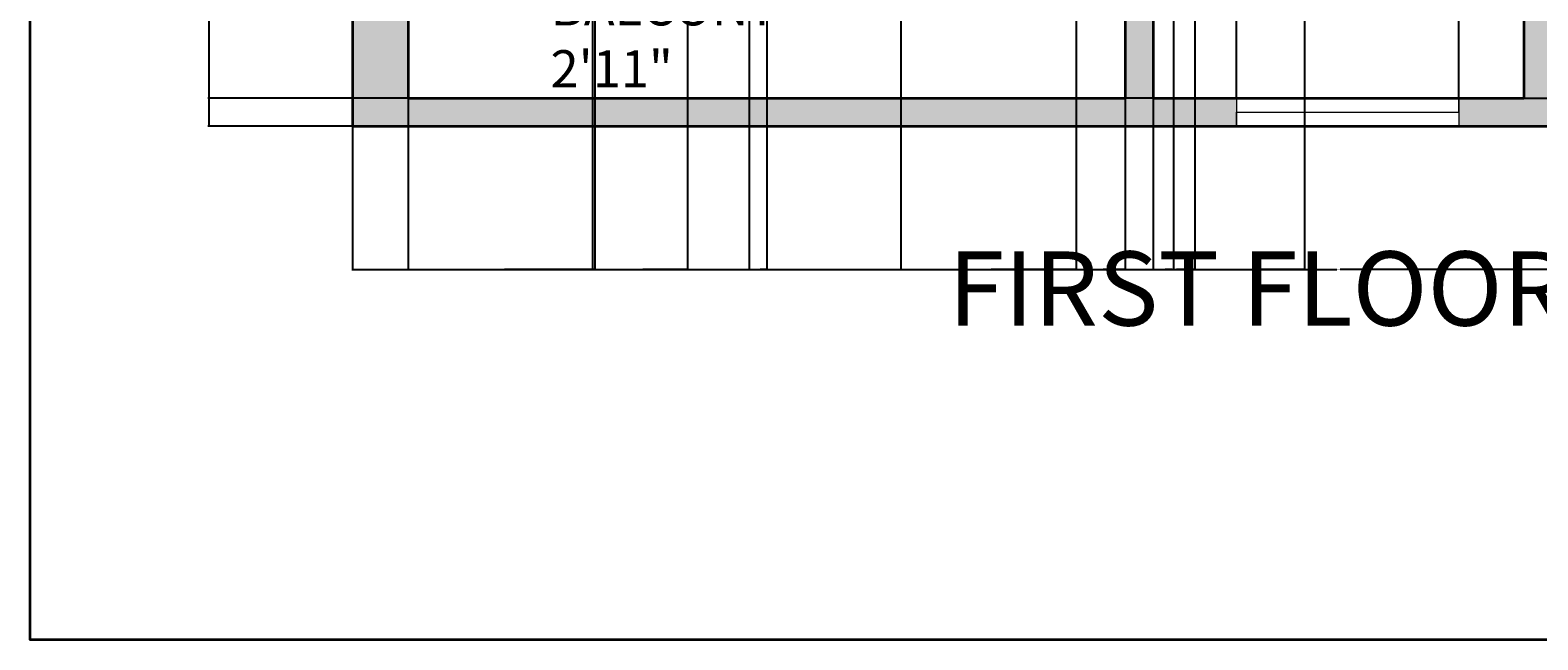
# Model space of a CAD drawing. Units: inches. Extents: x 2606 to 3027, y 1906 to 2463.
# Tile 1 of 10: x 2606 to 2850, y 1906 to 2004. Entities that reach past the tile are written whole.
import ezdxf

# ---------------------------------------------------------------- set-up
doc = ezdxf.new("R2010")
doc.units = ezdxf.units.IN
for name, color, linetype, lineweight in [('A-ANNO-DIMS', 2, 'Continuous', 18), ('A-ANNO-TEXT', 7, 'Continuous', 25), ('A-ANNO-TTLB', 7, 'Continuous', 35), ('A-AREA-IDEN', 7, 'Continuous', 18), ('A-GLAZ', 4, 'Continuous', 18), ('A-WALL', 7, 'Continuous', 35)]:
    doc.layers.add(name, color=color, linetype=linetype, lineweight=lineweight)
doc.layers.add('A-WALL-PATT', color=251, linetype='Continuous', lineweight=13, true_color=0x636466)
doc.styles.get("Standard").update_dxf_attribs({"font": 'arial.ttf'})
doc.dimstyles.get("Standard").update_dxf_attribs({"dimtxt": 0.18, "dimasz": 0.18, "dimexe": 0.18, "dimexo": 0.0625, "dimgap": 0.09, "dimtad": 0, "dimtih": 1, "dimtoh": 1, "dimdec": 4, "dimzin": 0, "dimdsep": 46, "dimtxsty": 'Standard', "dimcen": 0.09, "dimadec": 0, "dimazin": 0, "dimtfac": 1, "dimtdec": 4, "dimtofl": 0, "dimtmove": 0, "dimatfit": 3, "dimfxl": 1, "dimtolj": 1, "dimtzin": 0, "dimarcsym": 0})

# ---------------------------------------------------------------- blocks, each defined once
blk = doc.blocks.new('*D25')
at = {"layer": 'A-ANNO-DIMS', "color": 0, "lineweight": -2, "transparency": 16777216}
for p, q in [((2658.06, 1988.55), (2658.06, 1965.23)), ((2977.06, 1988.55), (2977.06, 1965.23)), ((2658.24, 1965.41), (2817.27, 1965.41)), ((2976.88, 1965.41), (2817.85, 1965.41))]:
    blk.add_line(p, q, dxfattribs=at)
at = {"layer": 'A-ANNO-DIMS', "color": 0, "transparency": 16777216}
for points in [[(2658.24, 1965.44), (2658.24, 1965.38), (2658.06, 1965.41)], [(2976.88, 1965.44), (2976.88, 1965.38), (2977.06, 1965.41)]]:
    blk.add_solid(points, dxfattribs=at)
at = {"layer": 'Defpoints', "color": 0, "transparency": 16777216}
for p in [(2658.06, 1988.61), (2977.06, 1988.61), (2977.06, 1965.41)]:
    blk.add_point(p, dxfattribs=at)
at = {"layer": 'A-ANNO-DIMS', "color": 0, "transparency": 16777216, "insert": (2817.56, 1965.41), "char_height": 0.18, "attachment_point": 5}
blk.add_mtext('\\A1;319', dxfattribs=at)
blk = doc.blocks.new('*D35')
at = {"layer": 'A-ANNO-DIMS', "color": 0, "lineweight": -2, "transparency": 16777216}
for p, q in [((2801.04, 1993.17), (2801.04, 2433.99)), ((2801.22, 2433.81), (2818.82, 2433.81)), ((2836.86, 2433.81), (2819.26, 2433.81)), ((2837.04, 1993.17), (2837.04, 2433.99))]:
    blk.add_line(p, q, dxfattribs=at)
at = {"layer": 'A-ANNO-DIMS', "color": 0, "transparency": 16777216}
for points in [[(2801.22, 2433.84), (2801.22, 2433.78), (2801.04, 2433.81)], [(2836.86, 2433.84), (2836.86, 2433.78), (2837.04, 2433.81)]]:
    blk.add_solid(points, dxfattribs=at)
at = {"layer": 'Defpoints', "color": 0, "transparency": 16777216}
for p in [(2837.04, 2433.81), (2801.04, 1993.11), (2837.04, 1993.11)]:
    blk.add_point(p, dxfattribs=at)
at = {"layer": 'A-ANNO-DIMS', "color": 0, "transparency": 16777216, "insert": (2819.04, 2433.81), "char_height": 0.18, "attachment_point": 5}
blk.add_mtext('\\A1;36', dxfattribs=at)
blk = doc.blocks.new('*D36')
at = {"layer": 'A-ANNO-DIMS', "color": 0, "lineweight": -2, "transparency": 16777216}
for p, q in [((2787.56, 1993.17), (2787.56, 2433.99)), ((2787.74, 2433.81), (2793.85, 2433.81)), ((2800.86, 2433.81), (2794.76, 2433.81)), ((2801.04, 1993.17), (2801.04, 2433.99))]:
    blk.add_line(p, q, dxfattribs=at)
at = {"layer": 'A-ANNO-DIMS', "color": 0, "transparency": 16777216}
for points in [[(2787.74, 2433.84), (2787.74, 2433.78), (2787.56, 2433.81)], [(2800.86, 2433.84), (2800.86, 2433.78), (2801.04, 2433.81)]]:
    blk.add_solid(points, dxfattribs=at)
at = {"layer": 'Defpoints', "color": 0, "transparency": 16777216}
for p in [(2787.56, 2433.81), (2787.56, 1993.11), (2801.04, 1993.11)]:
    blk.add_point(p, dxfattribs=at)
at = {"layer": 'A-ANNO-DIMS', "color": 0, "transparency": 16777216, "insert": (2794.3, 2433.81), "char_height": 0.18, "attachment_point": 5}
blk.add_mtext('\\A1;13.478', dxfattribs=at)
blk = doc.blocks.new('*D37')
at = {"layer": 'A-ANNO-DIMS', "color": 0, "lineweight": -2, "transparency": 16777216}
for p, q in [((2667, 2028.11), (2634.68, 2028.11)), ((2634.86, 2027.93), (2634.86, 2008.54)), ((2634.86, 1988.79), (2634.86, 2008.18)), ((2658, 1988.61), (2634.68, 1988.61))]:
    blk.add_line(p, q, dxfattribs=at)
at = {"layer": 'A-ANNO-DIMS', "color": 0, "transparency": 16777216}
for points in [[(2634.83, 2027.93), (2634.89, 2027.93), (2634.86, 2028.11)], [(2634.83, 1988.79), (2634.89, 1988.79), (2634.86, 1988.61)]]:
    blk.add_solid(points, dxfattribs=at)
at = {"layer": 'Defpoints', "color": 0, "transparency": 16777216}
for p in [(2634.86, 2028.11), (2667.06, 2028.11), (2658.06, 1988.61)]:
    blk.add_point(p, dxfattribs=at)
at = {"layer": 'A-ANNO-DIMS', "color": 0, "transparency": 16777216, "insert": (2634.86, 2008.36), "char_height": 0.18, "attachment_point": 5}
blk.add_mtext('\\A1;39.5', dxfattribs=at)
blk = doc.blocks.new('*D38')
at = {"layer": 'A-ANNO-DIMS', "color": 0, "lineweight": -2, "transparency": 16777216}
for p, q in [((2783.06, 1993.17), (2783.06, 2433.99)), ((2783.24, 2433.81), (2785.05, 2433.81)), ((2787.38, 2433.81), (2785.57, 2433.81)), ((2787.56, 1993.17), (2787.56, 2433.99))]:
    blk.add_line(p, q, dxfattribs=at)
at = {"layer": 'A-ANNO-DIMS', "color": 0, "transparency": 16777216}
for points in [[(2783.24, 2433.84), (2783.24, 2433.78), (2783.06, 2433.81)], [(2787.38, 2433.84), (2787.38, 2433.78), (2787.56, 2433.81)]]:
    blk.add_solid(points, dxfattribs=at)
at = {"layer": 'Defpoints', "color": 0, "transparency": 16777216}
for p in [(2787.56, 2433.81), (2783.06, 1993.11), (2787.56, 1993.11)]:
    blk.add_point(p, dxfattribs=at)
at = {"layer": 'A-ANNO-DIMS', "color": 0, "transparency": 16777216, "insert": (2785.31, 2433.81), "char_height": 0.18, "attachment_point": 5}
blk.add_mtext('\\A1;4.5', dxfattribs=at)
blk = doc.blocks.new('*D40')
at = {"layer": 'A-ANNO-DIMS', "color": 0, "lineweight": -2, "transparency": 16777216}
for p, q in [((2847.5, 2037.21), (2634.68, 2037.21)), ((2634.86, 2037.03), (2634.86, 2015.34)), ((2634.86, 1993.29), (2634.86, 2014.98)), ((2847.5, 1993.11), (2634.68, 1993.11))]:
    blk.add_line(p, q, dxfattribs=at)
at = {"layer": 'A-ANNO-DIMS', "color": 0, "transparency": 16777216}
for points in [[(2634.83, 2037.03), (2634.89, 2037.03), (2634.86, 2037.21)], [(2634.83, 1993.29), (2634.89, 1993.29), (2634.86, 1993.11)]]:
    blk.add_solid(points, dxfattribs=at)
at = {"layer": 'Defpoints', "color": 0, "transparency": 16777216}
for p in [(2847.56, 2037.21), (2634.86, 1993.11), (2847.56, 1993.11)]:
    blk.add_point(p, dxfattribs=at)
at = {"layer": 'A-ANNO-DIMS', "color": 0, "transparency": 16777216, "insert": (2634.86, 2015.16), "char_height": 0.18, "attachment_point": 5}
blk.add_mtext('\\A1;44.1', dxfattribs=at)
blk = doc.blocks.new('*D41')
at = {"layer": 'A-ANNO-DIMS', "color": 0, "lineweight": -2, "transparency": 16777216}
for p, q in [((2787.63, 2157.11), (3000.44, 2157.11)), ((3000.26, 2156.93), (3000.26, 2075.29)), ((3000.26, 1993.29), (3000.26, 2074.93)), ((2787.63, 1993.11), (3000.44, 1993.11))]:
    blk.add_line(p, q, dxfattribs=at)
at = {"layer": 'A-ANNO-DIMS', "color": 0, "transparency": 16777216}
for points in [[(3000.23, 2156.93), (3000.29, 2156.93), (3000.26, 2157.11)], [(3000.23, 1993.29), (3000.29, 1993.29), (3000.26, 1993.11)]]:
    blk.add_solid(points, dxfattribs=at)
at = {"layer": 'Defpoints', "color": 0, "transparency": 16777216}
for p in [(2787.56, 2157.11), (2787.56, 1993.11), (3000.26, 1993.11)]:
    blk.add_point(p, dxfattribs=at)
at = {"layer": 'A-ANNO-DIMS', "color": 0, "transparency": 16777216, "insert": (3000.26, 2075.11), "char_height": 0.18, "attachment_point": 5}
blk.add_mtext('\\A1;164', dxfattribs=at)
blk = doc.blocks.new('*D43')
at = {"layer": 'A-ANNO-DIMS', "color": 0, "lineweight": -2, "transparency": 16777216}
for p, q in [((2794.34, 2257.55), (2794.34, 1965.23)), ((2812.09, 2257.55), (2812.09, 1965.23)), ((2794.52, 1965.41), (2802.76, 1965.41)), ((2811.91, 1965.41), (2803.67, 1965.41))]:
    blk.add_line(p, q, dxfattribs=at)
at = {"layer": 'A-ANNO-DIMS', "color": 0, "transparency": 16777216}
for points in [[(2794.52, 1965.44), (2794.52, 1965.38), (2794.34, 1965.41)], [(2811.91, 1965.44), (2811.91, 1965.38), (2812.09, 1965.41)]]:
    blk.add_solid(points, dxfattribs=at)
at = {"layer": 'Defpoints', "color": 0, "transparency": 16777216}
for p in [(2794.34, 2257.61), (2812.09, 2257.61), (2812.09, 1965.41)]:
    blk.add_point(p, dxfattribs=at)
at = {"layer": 'A-ANNO-DIMS', "color": 0, "transparency": 16777216, "insert": (2803.22, 1965.41), "char_height": 0.18, "attachment_point": 5}
blk.add_mtext('\\A1;17.756', dxfattribs=at)
blk = doc.blocks.new('*D45')
at = {"layer": 'A-ANNO-DIMS', "color": 0, "lineweight": -2, "transparency": 16777216}
for p, q in [((2746.75, 2152.55), (2746.75, 1965.23)), ((2775.13, 2152.55), (2775.13, 1965.23)), ((2746.93, 1965.41), (2760.47, 1965.41)), ((2774.95, 1965.41), (2761.4, 1965.41))]:
    blk.add_line(p, q, dxfattribs=at)
at = {"layer": 'A-ANNO-DIMS', "color": 0, "transparency": 16777216}
for points in [[(2746.93, 1965.44), (2746.93, 1965.38), (2746.75, 1965.41)], [(2774.95, 1965.44), (2774.95, 1965.38), (2775.13, 1965.41)]]:
    blk.add_solid(points, dxfattribs=at)
at = {"layer": 'Defpoints', "color": 0, "transparency": 16777216}
for p in [(2746.75, 2152.61), (2775.13, 2152.61), (2775.13, 1965.41)]:
    blk.add_point(p, dxfattribs=at)
at = {"layer": 'A-ANNO-DIMS', "color": 0, "transparency": 16777216, "insert": (2760.94, 1965.41), "char_height": 0.18, "attachment_point": 5}
blk.add_mtext('\\A1;28.384', dxfattribs=at)
blk = doc.blocks.new('*D52')
at = {"layer": 'A-ANNO-DIMS', "color": 0, "lineweight": -2, "transparency": 16777216}
for p, q in [((2787.56, 2257.55), (2787.56, 1965.23)), ((2794.34, 2257.55), (2794.34, 1965.23)), ((2787.74, 1965.41), (2790.56, 1965.41)), ((2794.16, 1965.41), (2791.34, 1965.41))]:
    blk.add_line(p, q, dxfattribs=at)
at = {"layer": 'A-ANNO-DIMS', "color": 0, "transparency": 16777216}
for points in [[(2787.74, 1965.44), (2787.74, 1965.38), (2787.56, 1965.41)], [(2794.16, 1965.44), (2794.16, 1965.38), (2794.34, 1965.41)]]:
    blk.add_solid(points, dxfattribs=at)
at = {"layer": 'Defpoints', "color": 0, "transparency": 16777216}
for p in [(2787.56, 2257.61), (2794.34, 2257.61), (2794.34, 1965.41)]:
    blk.add_point(p, dxfattribs=at)
at = {"layer": 'A-ANNO-DIMS', "color": 0, "transparency": 16777216, "insert": (2790.95, 1965.41), "char_height": 0.18, "attachment_point": 5}
blk.add_mtext('\\A1;6.776', dxfattribs=at)
blk = doc.blocks.new('*D54')
at = {"layer": 'A-ANNO-DIMS', "color": 0, "lineweight": -2, "transparency": 16777216}
for p, q in [((2775.13, 2152.55), (2775.13, 1965.23)), ((2783.06, 2152.55), (2783.06, 1965.23)), ((2775.31, 1965.41), (2778.7, 1965.41)), ((2782.88, 1965.41), (2779.49, 1965.41))]:
    blk.add_line(p, q, dxfattribs=at)
at = {"layer": 'A-ANNO-DIMS', "color": 0, "transparency": 16777216}
for points in [[(2775.31, 1965.44), (2775.31, 1965.38), (2775.13, 1965.41)], [(2782.88, 1965.44), (2782.88, 1965.38), (2783.06, 1965.41)]]:
    blk.add_solid(points, dxfattribs=at)
at = {"layer": 'Defpoints', "color": 0, "transparency": 16777216}
for p in [(2775.13, 2152.61), (2783.06, 2152.61), (2783.06, 1965.41)]:
    blk.add_point(p, dxfattribs=at)
at = {"layer": 'A-ANNO-DIMS', "color": 0, "transparency": 16777216, "insert": (2779.1, 1965.41), "char_height": 0.18, "attachment_point": 5}
blk.add_mtext('\\A1;7.933', dxfattribs=at)
blk = doc.blocks.new('*D64')
at = {"layer": 'A-ANNO-DIMS', "color": 0, "lineweight": -2, "transparency": 16777216}
for p, q in [((2696.91, 2182.82), (2696.91, 1965.23)), ((2712.26, 2182.82), (2712.26, 1965.23)), ((2697.09, 1965.41), (2704.13, 1965.41)), ((2712.08, 1965.41), (2705.04, 1965.41))]:
    blk.add_line(p, q, dxfattribs=at)
at = {"layer": 'A-ANNO-DIMS', "color": 0, "transparency": 16777216}
for points in [[(2697.09, 1965.44), (2697.09, 1965.38), (2696.91, 1965.41)], [(2712.08, 1965.44), (2712.08, 1965.38), (2712.26, 1965.41)]]:
    blk.add_solid(points, dxfattribs=at)
at = {"layer": 'Defpoints', "color": 0, "transparency": 16777216}
for p in [(2696.91, 2182.88), (2712.26, 2182.88), (2712.26, 1965.41)]:
    blk.add_point(p, dxfattribs=at)
at = {"layer": 'A-ANNO-DIMS', "color": 0, "transparency": 16777216, "insert": (2704.58, 1965.41), "char_height": 0.18, "attachment_point": 5}
blk.add_mtext('\\A1;15.354', dxfattribs=at)
blk = doc.blocks.new('*D65')
at = {"layer": 'A-ANNO-DIMS', "color": 0, "lineweight": -2, "transparency": 16777216}
for p, q in [((2722.23, 2182.82), (2722.23, 1965.23)), ((2725.1, 2182.7), (2725.1, 1965.23)), ((2722.41, 1965.41), (2723.34, 1965.41)), ((2724.92, 1965.41), (2723.99, 1965.41))]:
    blk.add_line(p, q, dxfattribs=at)
at = {"layer": 'A-ANNO-DIMS', "color": 0, "transparency": 16777216}
for points in [[(2722.41, 1965.44), (2722.41, 1965.38), (2722.23, 1965.41)], [(2724.92, 1965.44), (2724.92, 1965.38), (2725.1, 1965.41)]]:
    blk.add_solid(points, dxfattribs=at)
at = {"layer": 'Defpoints', "color": 0, "transparency": 16777216}
for p in [(2722.23, 2182.88), (2725.1, 2182.76), (2725.1, 1965.41)]:
    blk.add_point(p, dxfattribs=at)
at = {"layer": 'A-ANNO-DIMS', "color": 0, "transparency": 16777216, "insert": (2723.66, 1965.41), "char_height": 0.18, "attachment_point": 5}
blk.add_mtext('\\A1;2.87', dxfattribs=at)
blk = doc.blocks.new('*D74')
at = {"layer": 'A-ANNO-DIMS', "color": 0, "lineweight": -2, "transparency": 16777216}
for p, q in [((2667.06, 2401.55), (2667.06, 1965.23)), ((2697.29, 2399.09), (2697.29, 1965.23)), ((2667.24, 1965.41), (2681.71, 1965.41)), ((2697.11, 1965.41), (2682.64, 1965.41))]:
    blk.add_line(p, q, dxfattribs=at)
at = {"layer": 'A-ANNO-DIMS', "color": 0, "transparency": 16777216}
for points in [[(2667.24, 1965.44), (2667.24, 1965.38), (2667.06, 1965.41)], [(2697.11, 1965.44), (2697.11, 1965.38), (2697.29, 1965.41)]]:
    blk.add_solid(points, dxfattribs=at)
at = {"layer": 'Defpoints', "color": 0, "transparency": 16777216}
for p in [(2667.06, 2401.61), (2697.29, 2399.15), (2667.06, 1965.41)]:
    blk.add_point(p, dxfattribs=at)
at = {"layer": 'A-ANNO-DIMS', "color": 0, "transparency": 16777216, "insert": (2682.18, 1965.41), "char_height": 0.18, "attachment_point": 5}
blk.add_mtext('\\A1;30.225', dxfattribs=at)
blk = doc.blocks.new('*D83')
at = {"layer": 'A-ANNO-DIMS', "color": 0, "lineweight": -2, "transparency": 16777216}
for p, q in [((2787.56, 2327.05), (2787.56, 1965.23)), ((2790.85, 2327.05), (2790.85, 1965.23)), ((2787.74, 1965.41), (2788.88, 1965.41)), ((2790.67, 1965.41), (2789.53, 1965.41))]:
    blk.add_line(p, q, dxfattribs=at)
at = {"layer": 'A-ANNO-DIMS', "color": 0, "transparency": 16777216}
for points in [[(2787.74, 1965.44), (2787.74, 1965.38), (2787.56, 1965.41)], [(2790.67, 1965.44), (2790.67, 1965.38), (2790.85, 1965.41)]]:
    blk.add_solid(points, dxfattribs=at)
at = {"layer": 'Defpoints', "color": 0, "transparency": 16777216}
for p in [(2787.56, 2327.11), (2790.85, 2327.11), (2790.85, 1965.41)]:
    blk.add_point(p, dxfattribs=at)
at = {"layer": 'A-ANNO-DIMS', "color": 0, "transparency": 16777216, "insert": (2789.21, 1965.41), "char_height": 0.18, "attachment_point": 5}
blk.add_mtext('\\A1;3.29', dxfattribs=at)

msp = doc.modelspace()

# ---------------------------------------------------------------- hatches: boundary and pattern name
at = {"layer": 'A-WALL-PATT'}
h = msp.add_hatch(color=256, dxfattribs=at)
h.dxf.hatch_style = 1
h.paths.add_polyline_path([(2667.063, 2401.6097), (2691.9697, 2401.6097), (2691.9697, 2406.1097), (2691.9697, 2410.6097), (2658.063, 2410.6097), (2658.063, 2238.7051), (2667.063, 2238.7051)])
h.paths.add_polyline_path([(2804.9965, 2406.1097), (2804.9965, 2410.6097), (2751.9697, 2410.6097), (2751.9697, 2401.6097), (2783.063, 2401.6097), (2783.063, 2257.6097), (2778.6739, 2257.6097), (2778.6739, 2253.1097), (2792.3386, 2253.1097), (2792.3386, 2255.3597), (2792.3386, 2257.6097), (2787.563, 2257.6097), (2787.563, 2327.1097), (2847.563, 2327.1097), (2847.563, 2331.6097), (2787.563, 2331.6097), (2787.563, 2401.6097), (2804.9965, 2401.6097)])
h.paths.add_polyline_path([(2889.6183, 2406.1097), (2889.6183, 2410.6097), (2828.9965, 2410.6097), (2828.9965, 2401.6097), (2831.8174, 2401.6097), (2847.563, 2401.6097), (2847.563, 2357.8311), (2849.813, 2357.8311), (2852.063, 2357.8311), (2852.063, 2401.6097), (2889.6183, 2401.6097)])
h.paths.add_polyline_path([(2977.063, 2410.6097), (2949.6183, 2410.6097), (2949.6183, 2401.6097), (2968.063, 2401.6097), (2968.063, 2157.1097), (2897.063, 2157.1097), (2897.063, 2174.1966), (2892.563, 2174.1966), (2892.563, 2157.1097), (2886.8122, 2157.1097), (2886.8122, 2152.6097), (2968.063, 2152.6097), (2968.063, 2032.6097), (2950.8911, 2032.6097), (2950.8911, 2028.1097), (2968.063, 2028.1097), (2968.063, 1993.1097), (2852.063, 1993.1097), (2852.063, 2028.1097), (2856.0743, 2028.1097), (2856.0743, 2030.3597), (2856.0743, 2032.6097), (2852.063, 2032.6097), (2852.063, 2152.6097), (2857.369, 2152.6097), (2857.369, 2154.8597), (2857.369, 2157.1097), (2847.563, 2157.1097), (2847.563, 2152.6097), (2847.563, 1993.1097), (2837.0415, 1993.1097), (2837.0415, 1988.6097), (2977.063, 1988.6097)])
h.paths.add_polyline_path([(2968.063, 2257.6097), (2886.9679, 2257.6097), (2886.9679, 2253.1097), (2892.563, 2253.1097), (2892.563, 2215.1332), (2897.063, 2215.1332), (2897.063, 2253.1097), (2968.063, 2253.1097)], flags=17)
h.paths.add_polyline_path([(2856.057, 2255.3597), (2856.057, 2257.6097), (2852.063, 2257.6097), (2852.063, 2336.7476), (2849.813, 2336.7476), (2847.563, 2336.7476), (2847.563, 2331.6097), (2847.563, 2327.1097), (2847.563, 2257.6097), (2813.482, 2257.6097), (2813.482, 2253.1097), (2856.057, 2253.1097)])
h.paths.add_polyline_path([(2748.8874, 2255.3597), (2748.8874, 2257.6097), (2667.063, 2257.6097), (2667.063, 2253.1097), (2748.8874, 2253.1097)])
h.paths.add_polyline_path([(2667.063, 2152.6097), (2744.8238, 2152.6097), (2744.8238, 2154.8597), (2744.8238, 2157.1097), (2667.063, 2157.1097), (2667.063, 2178.7051), (2658.063, 2178.7051), (2658.063, 1988.6097), (2801.0415, 1988.6097), (2801.0415, 1990.8597), (2801.0415, 1993.1097), (2787.563, 1993.1097), (2787.563, 2157.1097), (2777.1295, 2157.1097), (2777.1295, 2152.6097), (2783.063, 2152.6097), (2783.063, 2032.6097), (2778.4484, 2032.6097), (2778.4484, 2028.1097), (2783.063, 2028.1097), (2783.063, 1993.1097), (2667.063, 1993.1097), (2667.063, 2028.1097), (2680.1652, 2028.1097), (2680.1652, 2030.3597), (2680.1652, 2032.6097), (2667.063, 2032.6097)])
h.paths.add_polyline_path([(2755.4074, 2032.6097), (2728.1652, 2032.6097), (2728.1652, 2028.1097), (2755.4074, 2028.1097), (2755.4074, 2030.3597)], flags=17)
h.paths.add_polyline_path([(2902.8911, 2030.3597), (2902.8911, 2032.6097), (2877.6885, 2032.6097), (2877.6885, 2028.1097), (2902.8911, 2028.1097)], flags=17)
h.paths.add_polyline_path([(2810.2211, 2267.221), (2851.2716, 2267.221), (2851.2716, 2289.6098), (2810.2211, 2289.6098)], flags=9)

# ---------------------------------------------------------------- linework, layer by layer
at = {"layer": 'A-ANNO-TTLB'}
msp.add_lwpolyline([(2605.9227, 2462.7868), (3027.4339, 2462.7868), (3027.4339, 1905.5336), (2605.9227, 1905.5336)], close=True, dxfattribs=at)
at = {"layer": 'A-GLAZ'}
for p, q in [((2801.0415, 1993.1097), (2801.0415, 1988.6097)), ((2837.0415, 1990.8597), (2837.0415, 1993.1097)), ((2837.0415, 1993.1097), (2837.0415, 1988.6097)), ((2801.0415, 1988.6097), (2801.0415, 1990.8597)), ((2801.0415, 1990.8597), (2837.0415, 1990.8597))]:
    msp.add_line(p, q, dxfattribs=at)
at = {"layer": 'A-WALL'}
for p, q in [((2658.063, 2410.6097), (2658.063, 1988.6097)), ((2787.563, 2157.1097), (2787.563, 1993.1097)), ((2847.563, 2152.6097), (2847.563, 1993.1097)), ((2667.063, 2028.1097), (2667.063, 1993.1097)), ((2783.063, 2028.1097), (2783.063, 1993.1097)), ((2667.063, 1993.1097), (2783.063, 1993.1097)), ((2787.563, 1993.1097), (2847.563, 1993.1097)), ((2658.063, 1988.6097), (2977.063, 1988.6097))]:
    msp.add_line(p, q, dxfattribs=at)

# ---------------------------------------------------------------- texts
at = {"layer": 'A-ANNO-TEXT', "insert": (2754.4391, 1968.3416), "char_height": 12, "attachment_point": 1}
msp.add_mtext_dynamic_manual_height_columns('FIRST FLOOR PLAN', width=233.480418, gutter_width=12.5, heights=[0], dxfattribs=at)
at = {"layer": 'A-AREA-IDEN', "insert": (2690.1075, 2010.8806), "char_height": 6, "attachment_point": 1}
msp.add_mtext_dynamic_manual_height_columns('BALCONY\\P2\'11"', width=32.965259, gutter_width=12.5, heights=[0], dxfattribs=at)

# ---------------------------------------------------------------- dimensions: what is measured, and where the dimension line sits
at = {"layer": 'A-ANNO-DIMS'}
for base, p1, p2, override, picture, middle in [((2787.563, 2433.8097), (2783.063, 1993.1097), (2787.563, 1993.1097), {"dimdec": 1, "dimlfac": 1, "dimrnd": 0, "dimzin": 0, "dimdsep": 46, "dimlunit": 2}, '*D38', (2785.313, 2433.8097)), ((2787.56299, 2433.8097), (2801.04146, 1993.1097), (2787.56299, 1993.1097), {"dimdec": 3, "dimlfac": 1, "dimrnd": 0, "dimzin": 0, "dimdsep": 46, "dimlunit": 2}, '*D36', (2794.30223, 2433.8097)), ((2837.0415, 2433.8097), (2801.0415, 1993.1097), (2837.0415, 1993.1097), {"dimdec": 0, "dimlfac": 1, "dimrnd": 0, "dimzin": 0, "dimdsep": 46, "dimlunit": 2}, '*D35', (2819.0415, 2433.8097)), ((2667.063, 1965.4097), (2697.2878, 2399.1511), (2667.063, 2401.6097), {"dimdec": 3, "dimlfac": 1, "dimrnd": 0, "dimzin": 0, "dimdsep": 46, "dimlunit": 2}, '*D74', (2682.1754, 1965.4097)), ((2790.8496, 1965.4097), (2787.563, 2327.1097), (2790.8496, 2327.1097), {"dimdec": 2, "dimlfac": 1, "dimrnd": 0, "dimzin": 0, "dimdsep": 46, "dimlunit": 2}, '*D83', (2789.2063, 1965.4097)), ((2794.3386, 1965.4097), (2787.563, 2257.6097), (2794.3386, 2257.6097), {"dimdec": 3, "dimlfac": 1, "dimrnd": 0, "dimzin": 0, "dimdsep": 46, "dimlunit": 2}, '*D52', (2790.9508, 1965.4097)), ((2812.0947, 1965.4097), (2794.3386, 2257.6097), (2812.0947, 2257.6097), {"dimdec": 3, "dimlfac": 1, "dimrnd": 0, "dimzin": 0, "dimdsep": 46, "dimlunit": 2}, '*D43', (2803.2167, 1965.4097)), ((2712.2609, 1965.4097), (2696.9071, 2182.8782), (2712.2609, 2182.8782), {"dimdec": 3, "dimlfac": 1, "dimrnd": 0, "dimzin": 0, "dimdsep": 46, "dimlunit": 2}, '*D64', (2704.584, 1965.4097)), ((2725.1011, 1965.4097), (2722.2278, 2182.8782), (2725.1011, 2182.7588), {"dimdec": 2, "dimlfac": 1, "dimrnd": 0, "dimzin": 0, "dimdsep": 46, "dimlunit": 2}, '*D65', (2723.6644, 1965.4097)), ((2775.1295, 1965.4097), (2746.7452, 2152.6097), (2775.1295, 2152.6097), {"dimdec": 3, "dimlfac": 1, "dimrnd": 0, "dimzin": 0, "dimdsep": 46, "dimlunit": 2}, '*D45', (2760.9374, 1965.4097)), ((2783.06299, 1965.4097), (2775.12954, 2152.6097), (2783.06299, 2152.6097), {"dimdec": 3, "dimlfac": 1, "dimrnd": 0, "dimzin": 0, "dimdsep": 46, "dimlunit": 2}, '*D54', (2779.09627, 1965.4097)), ((2977.063, 1965.4097), (2658.063, 1988.6097), (2977.063, 1988.6097), {"dimdec": 0, "dimlfac": 1, "dimrnd": 0, "dimzin": 0, "dimdsep": 46, "dimlunit": 2}, '*D25', (2817.563, 1965.4097))]:
    dim = msp.add_linear_dim(base=base, p1=p1, p2=p2, dimstyle='Standard', override=override, dxfattribs=at)
    dim.commit()
    dim.dimension.update_dxf_attribs({"geometry": picture, "text_midpoint": middle})
for base, p1, p2, override, picture, middle in [((3000.263, 1993.1097), (2787.563, 2157.1097), (2787.563, 1993.1097), {"dimdec": 0, "dimlfac": 1, "dimrnd": 0, "dimzin": 0, "dimdsep": 46, "dimlunit": 2}, '*D41', (3000.263, 2075.1097)), ((2634.863, 1993.1097), (2847.563, 2037.2123), (2847.563, 1993.1097), {"dimdec": 1, "dimlfac": 1, "dimrnd": 0, "dimzin": 0, "dimdsep": 46, "dimlunit": 2}, '*D40', (2634.863, 2015.161)), ((2634.863, 2028.1097), (2658.063, 1988.6097), (2667.063, 2028.1097), {"dimdec": 1, "dimlfac": 1, "dimrnd": 0, "dimzin": 0, "dimdsep": 46, "dimlunit": 2}, '*D37', (2634.863, 2008.3597))]:
    dim = msp.add_linear_dim(base=base, p1=p1, p2=p2, angle=90, dimstyle='Standard', override=override, dxfattribs=at)
    dim.commit()
    dim.dimension.update_dxf_attribs({"geometry": picture, "text_midpoint": middle})

doc.saveas('drawing.dxf')
